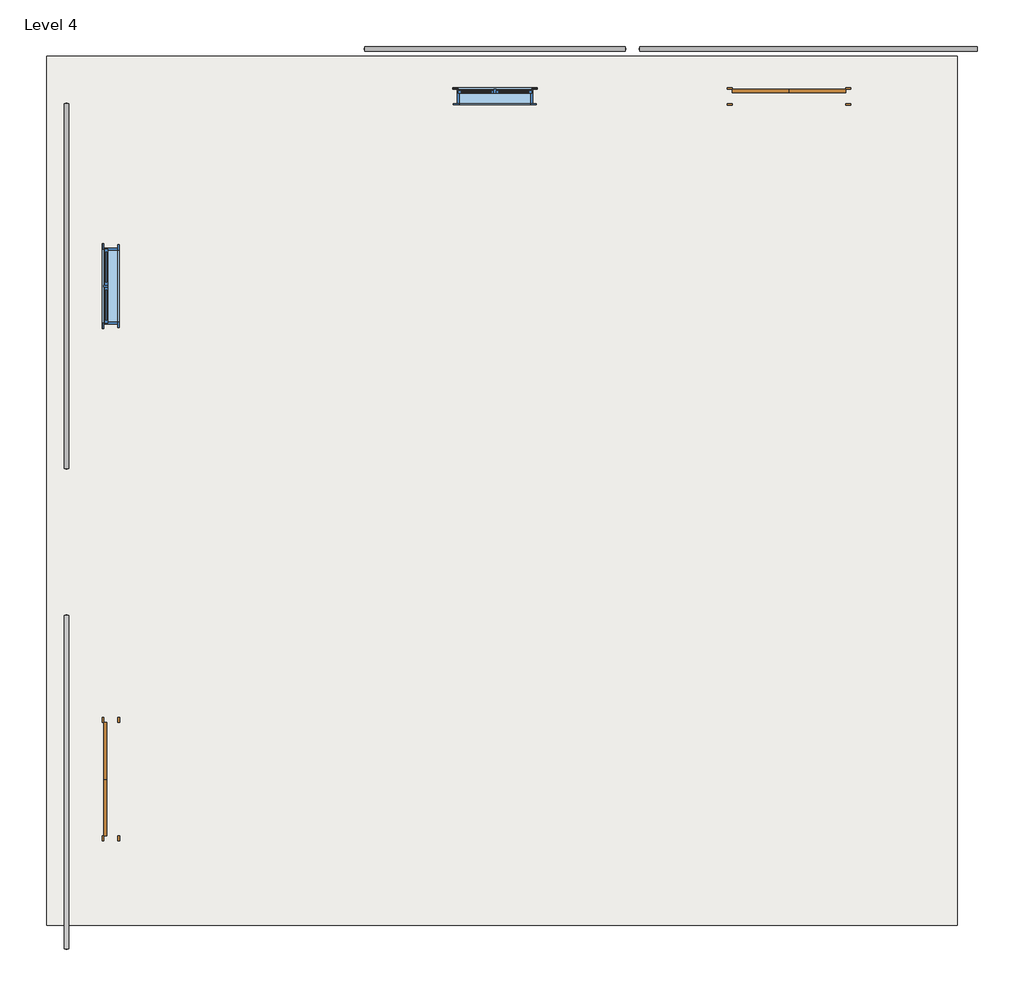
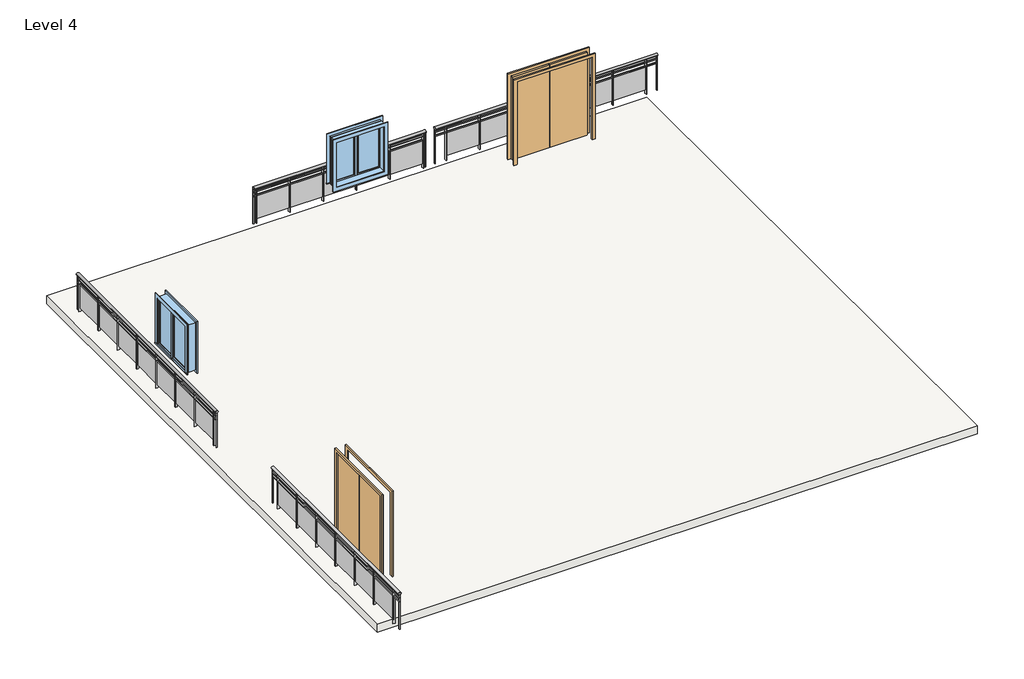
# One storey: 4 railings, 2 doors, 2 windows, 1 slab.
"""IFC4 building model written with IfcOpenShell, lengths in millimetres."""

from ifc_helpers import new_model, si_unit, point, frame, origin, place, context, project, spatial, polyline, ellipse_curve, trimmed, outline, extrude, transform, mapped, element, save
from ifc_brep_helpers import plane_surface, extruded_surface, advanced_brep
from components import door_640b4634, window_534dcd48

model = new_model("IFC4")

# Units and contexts
model_context = context("Model", 3, world=origin())
ifc_project = project(units=[si_unit("LENGTHUNIT", "METRE", prefix="MILLI")], contexts=[model_context])

# Site, building, storey
site = spatial("IfcSite", under=ifc_project)
building = spatial("IfcBuilding", under=site)
storey = spatial("IfcBuildingStorey", under=building, Name="Level 4", Elevation=9601.2)

# Doors
placement = place(None, origin())
door_shape = door_640b4634(model_context)
element("IfcDoor", 1, ObjectType="Door-Double-Flush_Panel : 72\" x 84\"", at=placement, inside=storey, context=model_context, shape_type="MappedRepresentation", body=[
    mapped(door_shape, transform((-18468.543393, -6784.3397804, 9601.2), x_axis=(0.0, 1.0, 0.0), y_axis=(-1.0, 0.0, 0.0), z_axis=(0.0, 0.0, 1.0))),
])
element("IfcDoor", 2, ObjectType="Door-Double-Flush_Panel : 72\" x 84\"", at=placement, inside=storey, context=model_context, shape_type="MappedRepresentation", body=[
    mapped(door_shape, transform((-7571.943393, 4188.4602196, 9601.2), x_axis=(1.0, 0.0, 0.0), y_axis=(0.0, 1.0, 0.0), z_axis=(0.0, 0.0, 1.0))),
])

# Railings
element("IfcRailing", 3, ObjectType="Glass Panel - Bottom Fill", at=placement, inside=storey, context=model_context, shape_type="SolidModel", body=[
    advanced_brep(
    [(-19220.0296876, -9514.8397804, 10515.6), (-19143.8296876, -9514.8397804, 10515.6), (-19220.0296876, -4155.4397804, 10515.6), (-19143.8296876, -4155.4397804, 10515.6)],
    [
        (0, 1, ellipse_curve(frame((-19181.9296876, -9514.8397804, 10515.6), z_axis=(0.0, -1.0, 0.0), x_axis=(1.0, 0.0, 0.0)), 38.1, 28.575)),
        (1, 0, ellipse_curve(frame((-19181.9296876, -9514.8397804, 10515.6), z_axis=(0.0, -1.0, 0.0), x_axis=(1.0, 0.0, 0.0)), 38.1, 28.575)),
        (2, 3, ellipse_curve(frame((-19181.9296876, -4155.4397804, 10515.6), z_axis=(0.0, 1.0, 0.0), x_axis=(1.0, 0.0, 0.0)), 38.1, 28.575)),
        (3, 2, ellipse_curve(frame((-19181.9296876, -4155.4397804, 10515.6), z_axis=(0.0, 1.0, 0.0), x_axis=(1.0, 0.0, 0.0)), 38.1, 28.575)),
        (0, 2),
        (3, 1),
    ],
    [
        plane_surface(frame((-19181.9296876, -9514.8397804, 10515.6), z_axis=(0.0, -1.0, 0.0), x_axis=(0.0, 0.0, 1.0))),
        plane_surface(frame((-19181.9296876, -4155.4397804, 10515.6), z_axis=(0.0, 1.0, 0.0), x_axis=(0.0, 0.0, 1.0))),
        extruded_surface(trimmed(ellipse_curve(frame((-19181.9296876, -4155.4397804, 10515.6), z_axis=(0.0, -1.0, 0.0), x_axis=(1.0, 0.0, 0.0)), 38.1, 28.575), [point((-19220.0296876, -4155.4397804, 10515.6))], [point((-19143.8296876, -4155.4397804, 10515.6))], True, "CARTESIAN"), (0.0, -5359.4, 0.0), 5359.4),
        extruded_surface(trimmed(ellipse_curve(frame((-19181.9296876, -4155.4397804, 10515.6), z_axis=(0.0, -1.0, 0.0), x_axis=(1.0, 0.0, 0.0)), 38.1, 28.575), [point((-19143.8296876, -4155.4397804, 10515.6))], [point((-19220.0296876, -4155.4397804, 10515.6))], True, "CARTESIAN"), (0.0, -5359.4, 0.0), 5359.4),
    ],
    [
        (0, [[1, 2]]),
        (1, [[3, 4]]),
        (2, [[-1, 5, -4, 6]]),
        (3, [[-2, -6, -3, -5]]),
    ],
),
    extrude(outline(polyline([(-19169.2296876, -9514.8397804), (-19194.6296876, -9514.8397804), (-19194.6296876, -4155.4397804), (-19169.2296876, -4155.4397804), (-19169.2296876, -9514.8397804)])), frame((0.0, 0.0, 10401.3), z_axis=(0.0, 0.0, 1.0), x_axis=(1.0, 0.0, 0.0)), (0.0, 0.0, 1.0), 25.4),
    extrude(outline(polyline([(-19169.2296876, -9514.8397804), (-19194.6296876, -9514.8397804), (-19194.6296876, -4155.4397804), (-19169.2296876, -4155.4397804), (-19169.2296876, -9514.8397804)])), frame((0.0, 0.0, 10299.7), z_axis=(0.0, 0.0, 1.0), x_axis=(1.0, 0.0, 0.0)), (0.0, 0.0, 1.0), 25.4),
    extrude(outline(polyline([(-19156.5296876, -4403.0897804), (-19207.3296876, -4403.0897804), (-19207.3296876, -4390.3897804), (-19156.5296876, -4390.3897804), (-19156.5296876, -4403.0897804)])), frame((0.0, 0.0, 9601.2), z_axis=(0.0, 0.0, 1.0), x_axis=(1.0, 0.0, 0.0)), (0.0, 0.0, 1.0), 885.6788223),
    extrude(outline(polyline([(-19188.4648446, -5209.5397804), (-19188.4648446, -4396.7397804), (-19182.1148446, -4396.7397804), (-19182.1148446, -5209.5397804), (-19188.4648446, -5209.5397804)])), frame((0.0, 0.0, 9702.8), z_axis=(0.0, 0.0, 1.0), x_axis=(1.0, 0.0, 0.0)), (0.0, 0.0, 1.0), 596.9),
    extrude(outline(polyline([(-19156.5296876, -5215.8897804), (-19207.3296876, -5215.8897804), (-19207.3296876, -5203.1897804), (-19156.5296876, -5203.1897804), (-19156.5296876, -5215.8897804)])), frame((0.0, 0.0, 9601.2), z_axis=(0.0, 0.0, 1.0), x_axis=(1.0, 0.0, 0.0)), (0.0, 0.0, 1.0), 885.6788223),
    extrude(outline(polyline([(-19188.4648446, -6022.3397804), (-19188.4648446, -5209.5397804), (-19182.1148446, -5209.5397804), (-19182.1148446, -6022.3397804), (-19188.4648446, -6022.3397804)])), frame((0.0, 0.0, 9702.8), z_axis=(0.0, 0.0, 1.0), x_axis=(1.0, 0.0, 0.0)), (0.0, 0.0, 1.0), 596.9),
    extrude(outline(polyline([(-19156.5296876, -6028.6897804), (-19207.3296876, -6028.6897804), (-19207.3296876, -6015.9897804), (-19156.5296876, -6015.9897804), (-19156.5296876, -6028.6897804)])), frame((0.0, 0.0, 9601.2), z_axis=(0.0, 0.0, 1.0), x_axis=(1.0, 0.0, 0.0)), (0.0, 0.0, 1.0), 885.6788223),
    extrude(outline(polyline([(-19188.4648446, -6835.1397804), (-19188.4648446, -6022.3397804), (-19182.1148446, -6022.3397804), (-19182.1148446, -6835.1397804), (-19188.4648446, -6835.1397804)])), frame((0.0, 0.0, 9702.8), z_axis=(0.0, 0.0, 1.0), x_axis=(1.0, 0.0, 0.0)), (0.0, 0.0, 1.0), 596.9),
    extrude(outline(polyline([(-19156.5296876, -6841.4897804), (-19207.3296876, -6841.4897804), (-19207.3296876, -6828.7897804), (-19156.5296876, -6828.7897804), (-19156.5296876, -6841.4897804)])), frame((0.0, 0.0, 9601.2), z_axis=(0.0, 0.0, 1.0), x_axis=(1.0, 0.0, 0.0)), (0.0, 0.0, 1.0), 885.6788223),
    extrude(outline(polyline([(-19188.4648446, -7647.9397804), (-19188.4648446, -6835.1397804), (-19182.1148446, -6835.1397804), (-19182.1148446, -7647.9397804), (-19188.4648446, -7647.9397804)])), frame((0.0, 0.0, 9702.8), z_axis=(0.0, 0.0, 1.0), x_axis=(1.0, 0.0, 0.0)), (0.0, 0.0, 1.0), 596.9),
    extrude(outline(polyline([(-19156.5296876, -7654.2897804), (-19207.3296876, -7654.2897804), (-19207.3296876, -7641.5897804), (-19156.5296876, -7641.5897804), (-19156.5296876, -7654.2897804)])), frame((0.0, 0.0, 9601.2), z_axis=(0.0, 0.0, 1.0), x_axis=(1.0, 0.0, 0.0)), (0.0, 0.0, 1.0), 885.6788223),
    extrude(outline(polyline([(-19188.4648446, -8460.7397804), (-19188.4648446, -7647.9397804), (-19182.1148446, -7647.9397804), (-19182.1148446, -8460.7397804), (-19188.4648446, -8460.7397804)])), frame((0.0, 0.0, 9702.8), z_axis=(0.0, 0.0, 1.0), x_axis=(1.0, 0.0, 0.0)), (0.0, 0.0, 1.0), 596.9),
    extrude(outline(polyline([(-19156.5296876, -8467.0897804), (-19207.3296876, -8467.0897804), (-19207.3296876, -8454.3897804), (-19156.5296876, -8454.3897804), (-19156.5296876, -8467.0897804)])), frame((0.0, 0.0, 9601.2), z_axis=(0.0, 0.0, 1.0), x_axis=(1.0, 0.0, 0.0)), (0.0, 0.0, 1.0), 885.6788223),
    extrude(outline(polyline([(-19188.4648446, -9273.5397804), (-19188.4648446, -8460.7397804), (-19182.1148446, -8460.7397804), (-19182.1148446, -9273.5397804), (-19188.4648446, -9273.5397804)])), frame((0.0, 0.0, 9702.8), z_axis=(0.0, 0.0, 1.0), x_axis=(1.0, 0.0, 0.0)), (0.0, 0.0, 1.0), 596.9),
    extrude(outline(polyline([(-19156.5296876, -9279.8897804), (-19207.3296876, -9279.8897804), (-19207.3296876, -9267.1897804), (-19156.5296876, -9267.1897804), (-19156.5296876, -9279.8897804)])), frame((0.0, 0.0, 9601.2), z_axis=(0.0, 0.0, 1.0), x_axis=(1.0, 0.0, 0.0)), (0.0, 0.0, 1.0), 885.6788223),
    extrude(outline(polyline([(-19172.4046876, -4168.1397804), (-19191.4546876, -4168.1397804), (-19191.4546876, -4149.0897804), (-19172.4046876, -4149.0897804), (-19172.4046876, -4168.1397804)])), frame((0.0, 0.0, 9601.2), z_axis=(0.0, 0.0, 1.0), x_axis=(1.0, 0.0, 0.0)), (0.0, 0.0, 1.0), 885.6788223),
    extrude(outline(polyline([(-19172.4046876, -9521.1897804), (-19191.4546876, -9521.1897804), (-19191.4546876, -9502.1397804), (-19172.4046876, -9502.1397804), (-19172.4046876, -9521.1897804)])), frame((0.0, 0.0, 9601.2), z_axis=(0.0, 0.0, 1.0), x_axis=(1.0, 0.0, 0.0)), (0.0, 0.0, 1.0), 885.6788223),
])
element("IfcRailing", 4, ObjectType="Glass Panel - Bottom Fill", at=placement, inside=storey, context=model_context, shape_type="SolidModel", body=[
    advanced_brep(
    [(-19143.8296876, 4074.1602196, 10515.6), (-19220.0296876, 4074.1602196, 10515.6), (-19143.8296876, -1793.2397804, 10515.6), (-19220.0296876, -1793.2397804, 10515.6)],
    [
        (0, 1, ellipse_curve(frame((-19181.9296876, 4074.1602196, 10515.6), z_axis=(0.0, 1.0, 0.0), x_axis=(-1.0, 0.0, 0.0)), 38.1, 28.575)),
        (1, 0, ellipse_curve(frame((-19181.9296876, 4074.1602196, 10515.6), z_axis=(0.0, 1.0, 0.0), x_axis=(-1.0, 0.0, 0.0)), 38.1, 28.575)),
        (2, 3, ellipse_curve(frame((-19181.9296876, -1793.2397804, 10515.6), z_axis=(0.0, -1.0, 0.0), x_axis=(-1.0, 0.0, 0.0)), 38.1, 28.575)),
        (3, 2, ellipse_curve(frame((-19181.9296876, -1793.2397804, 10515.6), z_axis=(0.0, -1.0, 0.0), x_axis=(-1.0, 0.0, 0.0)), 38.1, 28.575)),
        (0, 2),
        (3, 1),
    ],
    [
        plane_surface(frame((-19181.9296876, 4074.1602196, 10515.6), z_axis=(0.0, 1.0, 0.0), x_axis=(0.0, 0.0, -1.0))),
        plane_surface(frame((-19181.9296876, -1793.2397804, 10515.6), z_axis=(0.0, -1.0, 0.0), x_axis=(0.0, 0.0, -1.0))),
        extruded_surface(trimmed(ellipse_curve(frame((-19181.9296876, -1793.2397804, 10515.6), z_axis=(0.0, 1.0, 0.0), x_axis=(-1.0, 0.0, 0.0)), 38.1, 28.575), [point((-19143.8296876, -1793.2397804, 10515.6))], [point((-19220.0296876, -1793.2397804, 10515.6))], True, "CARTESIAN"), (0.0, 5867.4, 0.0), 5867.4),
        extruded_surface(trimmed(ellipse_curve(frame((-19181.9296876, -1793.2397804, 10515.6), z_axis=(0.0, 1.0, 0.0), x_axis=(-1.0, 0.0, 0.0)), 38.1, 28.575), [point((-19220.0296876, -1793.2397804, 10515.6))], [point((-19143.8296876, -1793.2397804, 10515.6))], True, "CARTESIAN"), (0.0, 5867.4, 0.0), 5867.4),
    ],
    [
        (0, [[1, 2]]),
        (1, [[3, 4]]),
        (2, [[-1, 5, -4, 6]]),
        (3, [[-2, -6, -3, -5]]),
    ],
),
    extrude(outline(polyline([(-19194.6296876, 4074.1602196), (-19169.2296876, 4074.1602196), (-19169.2296876, -1793.2397804), (-19194.6296876, -1793.2397804), (-19194.6296876, 4074.1602196)])), frame((0.0, 0.0, 10401.3), z_axis=(0.0, 0.0, 1.0), x_axis=(1.0, 0.0, 0.0)), (0.0, 0.0, 1.0), 25.4),
    extrude(outline(polyline([(-19194.6296876, 4074.1602196), (-19169.2296876, 4074.1602196), (-19169.2296876, -1793.2397804), (-19194.6296876, -1793.2397804), (-19194.6296876, 4074.1602196)])), frame((0.0, 0.0, 10299.7), z_axis=(0.0, 0.0, 1.0), x_axis=(1.0, 0.0, 0.0)), (0.0, 0.0, 1.0), 25.4),
    extrude(outline(polyline([(-19207.3296876, -1697.9897804), (-19156.5296876, -1697.9897804), (-19156.5296876, -1710.6897804), (-19207.3296876, -1710.6897804), (-19207.3296876, -1697.9897804)])), frame((0.0, 0.0, 9601.2), z_axis=(0.0, 0.0, 1.0), x_axis=(1.0, 0.0, 0.0)), (0.0, 0.0, 1.0), 885.6788223),
    extrude(outline(polyline([(-19175.3945306, -891.5397804), (-19175.3945306, -1704.3397804), (-19181.7445306, -1704.3397804), (-19181.7445306, -891.5397804), (-19175.3945306, -891.5397804)])), frame((0.0, 0.0, 9702.8), z_axis=(0.0, 0.0, 1.0), x_axis=(1.0, 0.0, 0.0)), (0.0, 0.0, 1.0), 596.9),
    extrude(outline(polyline([(-19207.3296876, -885.1897804), (-19156.5296876, -885.1897804), (-19156.5296876, -897.8897804), (-19207.3296876, -897.8897804), (-19207.3296876, -885.1897804)])), frame((0.0, 0.0, 9601.2), z_axis=(0.0, 0.0, 1.0), x_axis=(1.0, 0.0, 0.0)), (0.0, 0.0, 1.0), 885.6788223),
    extrude(outline(polyline([(-19175.3945306, -78.7397804), (-19175.3945306, -891.5397804), (-19181.7445306, -891.5397804), (-19181.7445306, -78.7397804), (-19175.3945306, -78.7397804)])), frame((0.0, 0.0, 9702.8), z_axis=(0.0, 0.0, 1.0), x_axis=(1.0, 0.0, 0.0)), (0.0, 0.0, 1.0), 596.9),
    extrude(outline(polyline([(-19207.3296876, -72.3897804), (-19156.5296876, -72.3897804), (-19156.5296876, -85.0897804), (-19207.3296876, -85.0897804), (-19207.3296876, -72.3897804)])), frame((0.0, 0.0, 9601.2), z_axis=(0.0, 0.0, 1.0), x_axis=(1.0, 0.0, 0.0)), (0.0, 0.0, 1.0), 885.6788223),
    extrude(outline(polyline([(-19175.3945306, 734.0602196), (-19175.3945306, -78.7397804), (-19181.7445306, -78.7397804), (-19181.7445306, 734.0602196), (-19175.3945306, 734.0602196)])), frame((0.0, 0.0, 9702.8), z_axis=(0.0, 0.0, 1.0), x_axis=(1.0, 0.0, 0.0)), (0.0, 0.0, 1.0), 596.9),
    extrude(outline(polyline([(-19207.3296876, 740.4102196), (-19156.5296876, 740.4102196), (-19156.5296876, 727.7102196), (-19207.3296876, 727.7102196), (-19207.3296876, 740.4102196)])), frame((0.0, 0.0, 9601.2), z_axis=(0.0, 0.0, 1.0), x_axis=(1.0, 0.0, 0.0)), (0.0, 0.0, 1.0), 885.6788223),
    extrude(outline(polyline([(-19175.3945306, 1546.8602196), (-19175.3945306, 734.0602196), (-19181.7445306, 734.0602196), (-19181.7445306, 1546.8602196), (-19175.3945306, 1546.8602196)])), frame((0.0, 0.0, 9702.8), z_axis=(0.0, 0.0, 1.0), x_axis=(1.0, 0.0, 0.0)), (0.0, 0.0, 1.0), 596.9),
    extrude(outline(polyline([(-19207.3296876, 1553.2102196), (-19156.5296876, 1553.2102196), (-19156.5296876, 1540.5102196), (-19207.3296876, 1540.5102196), (-19207.3296876, 1553.2102196)])), frame((0.0, 0.0, 9601.2), z_axis=(0.0, 0.0, 1.0), x_axis=(1.0, 0.0, 0.0)), (0.0, 0.0, 1.0), 885.6788223),
    extrude(outline(polyline([(-19175.3945306, 2359.6602196), (-19175.3945306, 1546.8602196), (-19181.7445306, 1546.8602196), (-19181.7445306, 2359.6602196), (-19175.3945306, 2359.6602196)])), frame((0.0, 0.0, 9702.8), z_axis=(0.0, 0.0, 1.0), x_axis=(1.0, 0.0, 0.0)), (0.0, 0.0, 1.0), 596.9),
    extrude(outline(polyline([(-19207.3296876, 2366.0102196), (-19156.5296876, 2366.0102196), (-19156.5296876, 2353.3102196), (-19207.3296876, 2353.3102196), (-19207.3296876, 2366.0102196)])), frame((0.0, 0.0, 9601.2), z_axis=(0.0, 0.0, 1.0), x_axis=(1.0, 0.0, 0.0)), (0.0, 0.0, 1.0), 885.6788223),
    extrude(outline(polyline([(-19175.3945306, 3172.4602196), (-19175.3945306, 2359.6602196), (-19181.7445306, 2359.6602196), (-19181.7445306, 3172.4602196), (-19175.3945306, 3172.4602196)])), frame((0.0, 0.0, 9702.8), z_axis=(0.0, 0.0, 1.0), x_axis=(1.0, 0.0, 0.0)), (0.0, 0.0, 1.0), 596.9),
    extrude(outline(polyline([(-19207.3296876, 3178.8102196), (-19156.5296876, 3178.8102196), (-19156.5296876, 3166.1102196), (-19207.3296876, 3166.1102196), (-19207.3296876, 3178.8102196)])), frame((0.0, 0.0, 9601.2), z_axis=(0.0, 0.0, 1.0), x_axis=(1.0, 0.0, 0.0)), (0.0, 0.0, 1.0), 885.6788223),
    extrude(outline(polyline([(-19175.3945306, 3985.2602196), (-19175.3945306, 3172.4602196), (-19181.7445306, 3172.4602196), (-19181.7445306, 3985.2602196), (-19175.3945306, 3985.2602196)])), frame((0.0, 0.0, 9702.8), z_axis=(0.0, 0.0, 1.0), x_axis=(1.0, 0.0, 0.0)), (0.0, 0.0, 1.0), 596.9),
    extrude(outline(polyline([(-19207.3296876, 3991.6102196), (-19156.5296876, 3991.6102196), (-19156.5296876, 3978.9102196), (-19207.3296876, 3978.9102196), (-19207.3296876, 3991.6102196)])), frame((0.0, 0.0, 9601.2), z_axis=(0.0, 0.0, 1.0), x_axis=(1.0, 0.0, 0.0)), (0.0, 0.0, 1.0), 885.6788223),
    extrude(outline(polyline([(-19191.4546876, -1780.5397804), (-19172.4046876, -1780.5397804), (-19172.4046876, -1799.5897804), (-19191.4546876, -1799.5897804), (-19191.4546876, -1780.5397804)])), frame((0.0, 0.0, 9601.2), z_axis=(0.0, 0.0, 1.0), x_axis=(1.0, 0.0, 0.0)), (0.0, 0.0, 1.0), 885.6788223),
    extrude(outline(polyline([(-19191.4546876, 4080.5102196), (-19172.4046876, 4080.5102196), (-19172.4046876, 4061.4602196), (-19191.4546876, 4061.4602196), (-19191.4546876, 4080.5102196)])), frame((0.0, 0.0, 9601.2), z_axis=(0.0, 0.0, 1.0), x_axis=(1.0, 0.0, 0.0)), (0.0, 0.0, 1.0), 885.6788223),
])
element("IfcRailing", 5, ObjectType="Glass Panel - Bottom Fill", at=placement, inside=storey, context=model_context, shape_type="SolidModel", body=[
    advanced_brep(
    [(-14391.843393, 4991.4940048, 10515.6), (-14391.843393, 4915.2940048, 10515.6), (-10200.843393, 4991.4940048, 10515.6), (-10200.843393, 4915.2940048, 10515.6)],
    [
        (0, 1, ellipse_curve(frame((-14391.843393, 4953.3940048, 10515.6), z_axis=(-1.0, 0.0, 0.0), x_axis=(0.0, -1.0, 0.0)), 38.1, 28.575)),
        (1, 0, ellipse_curve(frame((-14391.843393, 4953.3940048, 10515.6), z_axis=(-1.0, 0.0, 0.0), x_axis=(0.0, -1.0, 0.0)), 38.1, 28.575)),
        (2, 3, ellipse_curve(frame((-10200.843393, 4953.3940048, 10515.6), z_axis=(1.0, 0.0, 0.0), x_axis=(0.0, -1.0, 0.0)), 38.1, 28.575)),
        (3, 2, ellipse_curve(frame((-10200.843393, 4953.3940048, 10515.6), z_axis=(1.0, 0.0, 0.0), x_axis=(0.0, -1.0, 0.0)), 38.1, 28.575)),
        (0, 2),
        (3, 1),
    ],
    [
        plane_surface(frame((-14391.843393, 4953.3940048, 10515.6), z_axis=(-1.0, 0.0, 0.0), x_axis=(0.0, 1.0, 0.0))),
        plane_surface(frame((-10200.843393, 4953.3940048, 10515.6), z_axis=(1.0, 0.0, 0.0), x_axis=(0.0, 1.0, 0.0))),
        extruded_surface(trimmed(ellipse_curve(frame((-10200.843393, 4953.3940048, 10515.6), z_axis=(-1.0, 0.0, 0.0), x_axis=(0.0, -1.0, 0.0)), 38.1, 28.575), [point((-10200.843393, 4991.4940048, 10515.6))], [point((-10200.843393, 4915.2940048, 10515.6))], True, "CARTESIAN"), (-4191.0, 0.0, 0.0), 4191.0),
        extruded_surface(trimmed(ellipse_curve(frame((-10200.843393, 4953.3940048, 10515.6), z_axis=(-1.0, 0.0, 0.0), x_axis=(0.0, -1.0, 0.0)), 38.1, 28.575), [point((-10200.843393, 4915.2940048, 10515.6))], [point((-10200.843393, 4991.4940048, 10515.6))], True, "CARTESIAN"), (-4191.0, 0.0, 0.0), 4191.0),
    ],
    [
        (0, [[1, 2]]),
        (1, [[3, 4]]),
        (2, [[-1, 5, -4, 6]]),
        (3, [[-2, -6, -3, -5]]),
    ],
),
    extrude(outline(polyline([(-14391.843393, 4940.6940048), (-14391.843393, 4966.0940048), (-10200.843393, 4966.0940048), (-10200.843393, 4940.6940048), (-14391.843393, 4940.6940048)])), frame((0.0, 0.0, 10401.3), z_axis=(0.0, 0.0, 1.0), x_axis=(1.0, 0.0, 0.0)), (0.0, 0.0, 1.0), 25.4),
    extrude(outline(polyline([(-14391.843393, 4940.6940048), (-14391.843393, 4966.0940048), (-10200.843393, 4966.0940048), (-10200.843393, 4940.6940048), (-14391.843393, 4940.6940048)])), frame((0.0, 0.0, 10299.7), z_axis=(0.0, 0.0, 1.0), x_axis=(1.0, 0.0, 0.0)), (0.0, 0.0, 1.0), 25.4),
    extrude(outline(polyline([(-10270.693393, 4927.9940048), (-10270.693393, 4978.7940048), (-10257.993393, 4978.7940048), (-10257.993393, 4927.9940048), (-10270.693393, 4927.9940048)])), frame((0.0, 0.0, 9601.2), z_axis=(0.0, 0.0, 1.0), x_axis=(1.0, 0.0, 0.0)), (0.0, 0.0, 1.0), 885.6788223),
    extrude(outline(polyline([(-11077.143393, 4959.9291618), (-10264.343393, 4959.9291618), (-10264.343393, 4953.5791618), (-11077.143393, 4953.5791618), (-11077.143393, 4959.9291618)])), frame((0.0, 0.0, 9702.8), z_axis=(0.0, 0.0, 1.0), x_axis=(1.0, 0.0, 0.0)), (0.0, 0.0, 1.0), 596.9),
    extrude(outline(polyline([(-11083.493393, 4927.9940048), (-11083.493393, 4978.7940048), (-11070.793393, 4978.7940048), (-11070.793393, 4927.9940048), (-11083.493393, 4927.9940048)])), frame((0.0, 0.0, 9601.2), z_axis=(0.0, 0.0, 1.0), x_axis=(1.0, 0.0, 0.0)), (0.0, 0.0, 1.0), 885.6788223),
    extrude(outline(polyline([(-11889.943393, 4959.9291618), (-11077.143393, 4959.9291618), (-11077.143393, 4953.5791618), (-11889.943393, 4953.5791618), (-11889.943393, 4959.9291618)])), frame((0.0, 0.0, 9702.8), z_axis=(0.0, 0.0, 1.0), x_axis=(1.0, 0.0, 0.0)), (0.0, 0.0, 1.0), 596.9),
    extrude(outline(polyline([(-11896.293393, 4927.9940048), (-11896.293393, 4978.7940048), (-11883.593393, 4978.7940048), (-11883.593393, 4927.9940048), (-11896.293393, 4927.9940048)])), frame((0.0, 0.0, 9601.2), z_axis=(0.0, 0.0, 1.0), x_axis=(1.0, 0.0, 0.0)), (0.0, 0.0, 1.0), 885.6788223),
    extrude(outline(polyline([(-12702.743393, 4959.9291618), (-11889.943393, 4959.9291618), (-11889.943393, 4953.5791618), (-12702.743393, 4953.5791618), (-12702.743393, 4959.9291618)])), frame((0.0, 0.0, 9702.8), z_axis=(0.0, 0.0, 1.0), x_axis=(1.0, 0.0, 0.0)), (0.0, 0.0, 1.0), 596.9),
    extrude(outline(polyline([(-12709.093393, 4927.9940048), (-12709.093393, 4978.7940048), (-12696.393393, 4978.7940048), (-12696.393393, 4927.9940048), (-12709.093393, 4927.9940048)])), frame((0.0, 0.0, 9601.2), z_axis=(0.0, 0.0, 1.0), x_axis=(1.0, 0.0, 0.0)), (0.0, 0.0, 1.0), 885.6788223),
    extrude(outline(polyline([(-13515.543393, 4959.9291618), (-12702.743393, 4959.9291618), (-12702.743393, 4953.5791618), (-13515.543393, 4953.5791618), (-13515.543393, 4959.9291618)])), frame((0.0, 0.0, 9702.8), z_axis=(0.0, 0.0, 1.0), x_axis=(1.0, 0.0, 0.0)), (0.0, 0.0, 1.0), 596.9),
    extrude(outline(polyline([(-13521.893393, 4927.9940048), (-13521.893393, 4978.7940048), (-13509.193393, 4978.7940048), (-13509.193393, 4927.9940048), (-13521.893393, 4927.9940048)])), frame((0.0, 0.0, 9601.2), z_axis=(0.0, 0.0, 1.0), x_axis=(1.0, 0.0, 0.0)), (0.0, 0.0, 1.0), 885.6788223),
    extrude(outline(polyline([(-14328.343393, 4959.9291618), (-13515.543393, 4959.9291618), (-13515.543393, 4953.5791618), (-14328.343393, 4953.5791618), (-14328.343393, 4959.9291618)])), frame((0.0, 0.0, 9702.8), z_axis=(0.0, 0.0, 1.0), x_axis=(1.0, 0.0, 0.0)), (0.0, 0.0, 1.0), 596.9),
    extrude(outline(polyline([(-14334.693393, 4927.9940048), (-14334.693393, 4978.7940048), (-14321.993393, 4978.7940048), (-14321.993393, 4927.9940048), (-14334.693393, 4927.9940048)])), frame((0.0, 0.0, 9601.2), z_axis=(0.0, 0.0, 1.0), x_axis=(1.0, 0.0, 0.0)), (0.0, 0.0, 1.0), 885.6788223),
    extrude(outline(polyline([(-10213.543393, 4943.8690048), (-10213.543393, 4962.9190048), (-10194.493393, 4962.9190048), (-10194.493393, 4943.8690048), (-10213.543393, 4943.8690048)])), frame((0.0, 0.0, 9601.2), z_axis=(0.0, 0.0, 1.0), x_axis=(1.0, 0.0, 0.0)), (0.0, 0.0, 1.0), 885.6788223),
    extrude(outline(polyline([(-14398.193393, 4943.8690048), (-14398.193393, 4962.9190048), (-14379.143393, 4962.9190048), (-14379.143393, 4943.8690048), (-14398.193393, 4943.8690048)])), frame((0.0, 0.0, 9601.2), z_axis=(0.0, 0.0, 1.0), x_axis=(1.0, 0.0, 0.0)), (0.0, 0.0, 1.0), 885.6788223),
])
element("IfcRailing", 6, ObjectType="Glass Panel - Bottom Fill", at=placement, inside=storey, context=model_context, shape_type="SolidModel", body=[
    advanced_brep(
    [(-9972.243393, 4991.4940048, 10515.6), (-9972.243393, 4915.2940048, 10515.6), (-4551.5296876, 4991.4940048, 10515.6), (-4551.5296876, 4915.2940048, 10515.6)],
    [
        (0, 1, ellipse_curve(frame((-9972.243393, 4953.3940048, 10515.6), z_axis=(-1.0, 0.0, 0.0), x_axis=(0.0, -1.0, 0.0)), 38.1, 28.575)),
        (1, 0, ellipse_curve(frame((-9972.243393, 4953.3940048, 10515.6), z_axis=(-1.0, 0.0, 0.0), x_axis=(0.0, -1.0, 0.0)), 38.1, 28.575)),
        (2, 3, ellipse_curve(frame((-4551.5296876, 4953.3940048, 10515.6), z_axis=(1.0, 0.0, 0.0), x_axis=(0.0, -1.0, 0.0)), 38.1, 28.575)),
        (3, 2, ellipse_curve(frame((-4551.5296876, 4953.3940048, 10515.6), z_axis=(1.0, 0.0, 0.0), x_axis=(0.0, -1.0, 0.0)), 38.1, 28.575)),
        (0, 2),
        (3, 1),
    ],
    [
        plane_surface(frame((-9972.243393, 4953.3940048, 10515.6), z_axis=(-1.0, 0.0, 0.0), x_axis=(0.0, 1.0, 0.0))),
        plane_surface(frame((-4551.5296876, 4953.3940048, 10515.6), z_axis=(1.0, 0.0, 0.0), x_axis=(0.0, 1.0, 0.0))),
        extruded_surface(trimmed(ellipse_curve(frame((-4551.5296876, 4953.3940048, 10515.6), z_axis=(-1.0, 0.0, 0.0), x_axis=(0.0, -1.0, 0.0)), 38.1, 28.575), [point((-4551.5296876, 4991.4940048, 10515.6))], [point((-4551.5296876, 4915.2940048, 10515.6))], True, "CARTESIAN"), (-5420.7137054, 0.0, 0.0), 5420.7137054),
        extruded_surface(trimmed(ellipse_curve(frame((-4551.5296876, 4953.3940048, 10515.6), z_axis=(-1.0, 0.0, 0.0), x_axis=(0.0, -1.0, 0.0)), 38.1, 28.575), [point((-4551.5296876, 4915.2940048, 10515.6))], [point((-4551.5296876, 4991.4940048, 10515.6))], True, "CARTESIAN"), (-5420.7137054, 0.0, 0.0), 5420.7137054),
    ],
    [
        (0, [[1, 2]]),
        (1, [[3, 4]]),
        (2, [[-1, 5, -4, 6]]),
        (3, [[-2, -6, -3, -5]]),
    ],
),
    extrude(outline(polyline([(-9972.243393, 4940.6940048), (-9972.243393, 4966.0940048), (-4551.5296876, 4966.0940048), (-4551.5296876, 4940.6940048), (-9972.243393, 4940.6940048)])), frame((0.0, 0.0, 10401.3), z_axis=(0.0, 0.0, 1.0), x_axis=(1.0, 0.0, 0.0)), (0.0, 0.0, 1.0), 25.4),
    extrude(outline(polyline([(-9972.243393, 4940.6940048), (-9972.243393, 4966.0940048), (-4551.5296876, 4966.0940048), (-4551.5296876, 4940.6940048), (-9972.243393, 4940.6940048)])), frame((0.0, 0.0, 10299.7), z_axis=(0.0, 0.0, 1.0), x_axis=(1.0, 0.0, 0.0)), (0.0, 0.0, 1.0), 25.4),
    extrude(outline(polyline([(-4829.8365403, 4927.9940048), (-4829.8365403, 4978.7940048), (-4817.1365403, 4978.7940048), (-4817.1365403, 4927.9940048), (-4829.8365403, 4927.9940048)])), frame((0.0, 0.0, 9601.2), z_axis=(0.0, 0.0, 1.0), x_axis=(1.0, 0.0, 0.0)), (0.0, 0.0, 1.0), 885.6788223),
    extrude(outline(polyline([(-5636.2865403, 4959.9291618), (-4823.4865403, 4959.9291618), (-4823.4865403, 4953.5791618), (-5636.2865403, 4953.5791618), (-5636.2865403, 4959.9291618)])), frame((0.0, 0.0, 9702.8), z_axis=(0.0, 0.0, 1.0), x_axis=(1.0, 0.0, 0.0)), (0.0, 0.0, 1.0), 596.9),
    extrude(outline(polyline([(-5642.6365403, 4927.9940048), (-5642.6365403, 4978.7940048), (-5629.9365403, 4978.7940048), (-5629.9365403, 4927.9940048), (-5642.6365403, 4927.9940048)])), frame((0.0, 0.0, 9601.2), z_axis=(0.0, 0.0, 1.0), x_axis=(1.0, 0.0, 0.0)), (0.0, 0.0, 1.0), 885.6788223),
    extrude(outline(polyline([(-6449.0865403, 4959.9291618), (-5636.2865403, 4959.9291618), (-5636.2865403, 4953.5791618), (-6449.0865403, 4953.5791618), (-6449.0865403, 4959.9291618)])), frame((0.0, 0.0, 9702.8), z_axis=(0.0, 0.0, 1.0), x_axis=(1.0, 0.0, 0.0)), (0.0, 0.0, 1.0), 596.9),
    extrude(outline(polyline([(-6455.4365403, 4927.9940048), (-6455.4365403, 4978.7940048), (-6442.7365403, 4978.7940048), (-6442.7365403, 4927.9940048), (-6455.4365403, 4927.9940048)])), frame((0.0, 0.0, 9601.2), z_axis=(0.0, 0.0, 1.0), x_axis=(1.0, 0.0, 0.0)), (0.0, 0.0, 1.0), 885.6788223),
    extrude(outline(polyline([(-7261.8865403, 4959.9291618), (-6449.0865403, 4959.9291618), (-6449.0865403, 4953.5791618), (-7261.8865403, 4953.5791618), (-7261.8865403, 4959.9291618)])), frame((0.0, 0.0, 9702.8), z_axis=(0.0, 0.0, 1.0), x_axis=(1.0, 0.0, 0.0)), (0.0, 0.0, 1.0), 596.9),
    extrude(outline(polyline([(-7268.2365403, 4927.9940048), (-7268.2365403, 4978.7940048), (-7255.5365403, 4978.7940048), (-7255.5365403, 4927.9940048), (-7268.2365403, 4927.9940048)])), frame((0.0, 0.0, 9601.2), z_axis=(0.0, 0.0, 1.0), x_axis=(1.0, 0.0, 0.0)), (0.0, 0.0, 1.0), 885.6788223),
    extrude(outline(polyline([(-8074.6865403, 4959.9291618), (-7261.8865403, 4959.9291618), (-7261.8865403, 4953.5791618), (-8074.6865403, 4953.5791618), (-8074.6865403, 4959.9291618)])), frame((0.0, 0.0, 9702.8), z_axis=(0.0, 0.0, 1.0), x_axis=(1.0, 0.0, 0.0)), (0.0, 0.0, 1.0), 596.9),
    extrude(outline(polyline([(-8081.0365403, 4927.9940048), (-8081.0365403, 4978.7940048), (-8068.3365403, 4978.7940048), (-8068.3365403, 4927.9940048), (-8081.0365403, 4927.9940048)])), frame((0.0, 0.0, 9601.2), z_axis=(0.0, 0.0, 1.0), x_axis=(1.0, 0.0, 0.0)), (0.0, 0.0, 1.0), 885.6788223),
    extrude(outline(polyline([(-8887.4865403, 4959.9291618), (-8074.6865403, 4959.9291618), (-8074.6865403, 4953.5791618), (-8887.4865403, 4953.5791618), (-8887.4865403, 4959.9291618)])), frame((0.0, 0.0, 9702.8), z_axis=(0.0, 0.0, 1.0), x_axis=(1.0, 0.0, 0.0)), (0.0, 0.0, 1.0), 596.9),
    extrude(outline(polyline([(-8893.8365403, 4927.9940048), (-8893.8365403, 4978.7940048), (-8881.1365403, 4978.7940048), (-8881.1365403, 4927.9940048), (-8893.8365403, 4927.9940048)])), frame((0.0, 0.0, 9601.2), z_axis=(0.0, 0.0, 1.0), x_axis=(1.0, 0.0, 0.0)), (0.0, 0.0, 1.0), 885.6788223),
    extrude(outline(polyline([(-9700.2865403, 4959.9291618), (-8887.4865403, 4959.9291618), (-8887.4865403, 4953.5791618), (-9700.2865403, 4953.5791618), (-9700.2865403, 4959.9291618)])), frame((0.0, 0.0, 9702.8), z_axis=(0.0, 0.0, 1.0), x_axis=(1.0, 0.0, 0.0)), (0.0, 0.0, 1.0), 596.9),
    extrude(outline(polyline([(-9706.6365403, 4927.9940048), (-9706.6365403, 4978.7940048), (-9693.9365403, 4978.7940048), (-9693.9365403, 4927.9940048), (-9706.6365403, 4927.9940048)])), frame((0.0, 0.0, 9601.2), z_axis=(0.0, 0.0, 1.0), x_axis=(1.0, 0.0, 0.0)), (0.0, 0.0, 1.0), 885.6788223),
    extrude(outline(polyline([(-4564.2296876, 4943.8690048), (-4564.2296876, 4962.9190048), (-4545.1796876, 4962.9190048), (-4545.1796876, 4943.8690048), (-4564.2296876, 4943.8690048)])), frame((0.0, 0.0, 9601.2), z_axis=(0.0, 0.0, 1.0), x_axis=(1.0, 0.0, 0.0)), (0.0, 0.0, 1.0), 885.6788223),
    extrude(outline(polyline([(-9978.593393, 4943.8690048), (-9978.593393, 4962.9190048), (-9959.543393, 4962.9190048), (-9959.543393, 4943.8690048), (-9978.593393, 4943.8690048)])), frame((0.0, 0.0, 9601.2), z_axis=(0.0, 0.0, 1.0), x_axis=(1.0, 0.0, 0.0)), (0.0, 0.0, 1.0), 885.6788223),
])

# Slab
element("IfcSlab", 7, ObjectType="Generic - 12\"", at=placement, inside=storey, context=model_context, shape_type="SweptSolid", body=[
    extrude(outline(polyline([(-4870.7979295, 4839.2351406), (-4870.7979295, -9131.9427484), (-19501.1979295, -9131.9427484), (-19501.1979295, 4839.2351406), (-4870.7979295, 4839.2351406)])), frame((0.0, 0.0, 9398.0), z_axis=(0.0, 0.0, 1.0), x_axis=(1.0, 0.0, 0.0)), (0.0, 0.0, 1.0), 203.2),
])

# Windows
window_shape = window_534dcd48(model_context)
element("IfcWindow", 8, ObjectType="Casement Dbl with Trim : 48\" x 48\"", at=placement, inside=storey, context=model_context, shape_type="MappedRepresentation", body=[
    mapped(window_shape, transform((-18449.493393, 1140.4602196, 8986.2811016), x_axis=(0.0, 1.0, 0.0), y_axis=(-1.0, 0.0, 0.0), z_axis=(0.0, 0.0, 1.0))),
])
element("IfcWindow", 9, ObjectType="Casement Dbl with Trim : 48\" x 48\"", at=placement, inside=storey, context=model_context, shape_type="MappedRepresentation", body=[
    mapped(window_shape, transform((-12296.343393, 4169.4102196, 9601.2), x_axis=(1.0, 0.0, 0.0), y_axis=(0.0, 1.0, 0.0), z_axis=(0.0, 0.0, 1.0))),
])

save(model, "model.ifc")

# Revit data of these elements
# Type "Door-Double-Flush_Panel : 72\" x 84\""
#   Type Mark = "11"
#   Construction Type Id = "DOOR"
#   Assembly Code = "C1020"
#   Analytic Construction = "Wooden"
#   Thickness = 0' - 2"
#   Thermal Resistance (R) = 2.5876 (h·ft²·°F)/BTU
#   Swing Angle [instance default] = 90.00°
#   Panel Width = 3' - 0"
#   Heat Transfer Coefficient (U) = 0.3865 BTU/(h·ft²·°F)
#   Height = 7' - 0"
#   Trim Projection Ext = 0' - 1"
#   Trim Projection Int = 0' - 1"
#   Trim Width = 0' - 3"
#   Width = 6' - 0"
#   Define Thermal Properties by = 1
#   Panel Material = Glass, Clear Glazing
#   Trim Material = Paint - Sienna
#   Visual Light Transmittance = 0
#   Solar Heat Gain Coefficient = 0
#   Function = (empty or 0)
#   Wall Closure = (empty or 0)
# Type "Glass Panel - Bottom Fill"
#   Assembly Code = "C2010400"
#   built-in parameter 1008612 = 0.0416667 (stored number, unit not read)
#   built-in parameter 1008611 = 0.0416667 (stored number, unit not read)
#   built-in parameter 1008609 = 0.333333 (stored number, unit not read)
#   built-in parameter 1008604 = 0.166667 (stored number, unit not read)
#   built-in parameter 1008603 = 0.166667 (stored number, unit not read)
#   Railing Height = 3' - 0"
#   built-in parameter 1008630 = 2
#   built-in parameter 1008610 = 2
#   built-in parameter 1008618 = Baluster - Square : 3/4"
# Type "Generic - 12\""
#   Assembly Code = "B1010"
#   Function = 0
#   Layers, outside or top first: 0' - 8" no material (function 1)
# Type "Casement Dbl with Trim : 48\" x 48\""
#   Type Mark = "10"
#   Construction Type Id = "GSP4R"
#   Assembly Code = "B2020100"
#   Analytic Construction = "1/8 in Pilkington single glazing"
#   Visual Light Transmittance = 0.9
#   Solar Heat Gain Coefficient = 0.78
#   Heat Transfer Coefficient (U) = 0.6496 BTU/(h·ft²·°F)
#   Height = 4' - 0"
#   Default Sill Height = 3' - 0"
#   Trim Projection - Ext. = 0' - 0 1/2"
#   Trim Projection - Int. = 0' - 0 3/4"
#   Trim Width - Exterior = 0' - 3 1/2"
#   Trim Width - Interior = 0' - 3 1/2"
#   Width = 4' - 0"
#   Window Inset = 0' - 0 3/4"
#   Define Thermal Properties by = 1
#   Glass Pane Material = Glass
#   Sash Material = Glass, Clear Glazing
#   Trim Exterior Material = Earth
#   Trim Interior Material = Trim
#   Wall Closure = (empty or 0)
# Elements 1, 2 (IfcDoor, "Door-Double-Flush_Panel : 72\" x 84\"")
#   Swing Angle = 90.00°
#   Phase Created = New Construction
#   Materials on its faces: "Paint - Sienna", "Glass, Clear Glazing"
# Elements 3, 4, 5, 6 (IfcRailing, "Glass Panel - Bottom Fill")
#   Phase Created = New Construction
#   Materials on its faces: "Glass"
# Element 7 (IfcSlab, "Generic - 12\"")
#   Height Offset From Level = 0' - 0"
#   Phase Created = New Construction
#   Materials on its faces: "Default Floor"
# Element 8 (IfcWindow, "Casement Dbl with Trim : 48\" x 48\"")
#   Mark = "3"
#   Phase Created = New Construction
#   Materials on its faces: "Glass, Clear Glazing", "Earth", "Glass", "Trim"
# Element 9 (IfcWindow, "Casement Dbl with Trim : 48\" x 48\"")
#   Mark = "6"
#   Phase Created = New Construction
#   Materials on its faces: "Glass, Clear Glazing", "Earth", "Glass", "Trim"
# Materials
#   "Glass, Clear Glazing": class "Glass", colour RGB 0 128 192, transparency 0.75, Description = "Clear glazing", Cost = 0
#   "Paint - Sienna": colour RGB 118 70 51, transparency 0, Cost = 0
#   "Glass": class "Glass", colour RGB 0 128 192, transparency 0.75, Description = "Soda Lime Glass", Cost = 0
#   "Earth": class "Generic", colour RGB 97 75 62, transparency 0, Description = "Soil", Cost = 0
#   "Trim": class "Wood", colour RGB 224 178 126, transparency 0
#   "Default Floor": colour RGB 128 128 128, transparency 0
